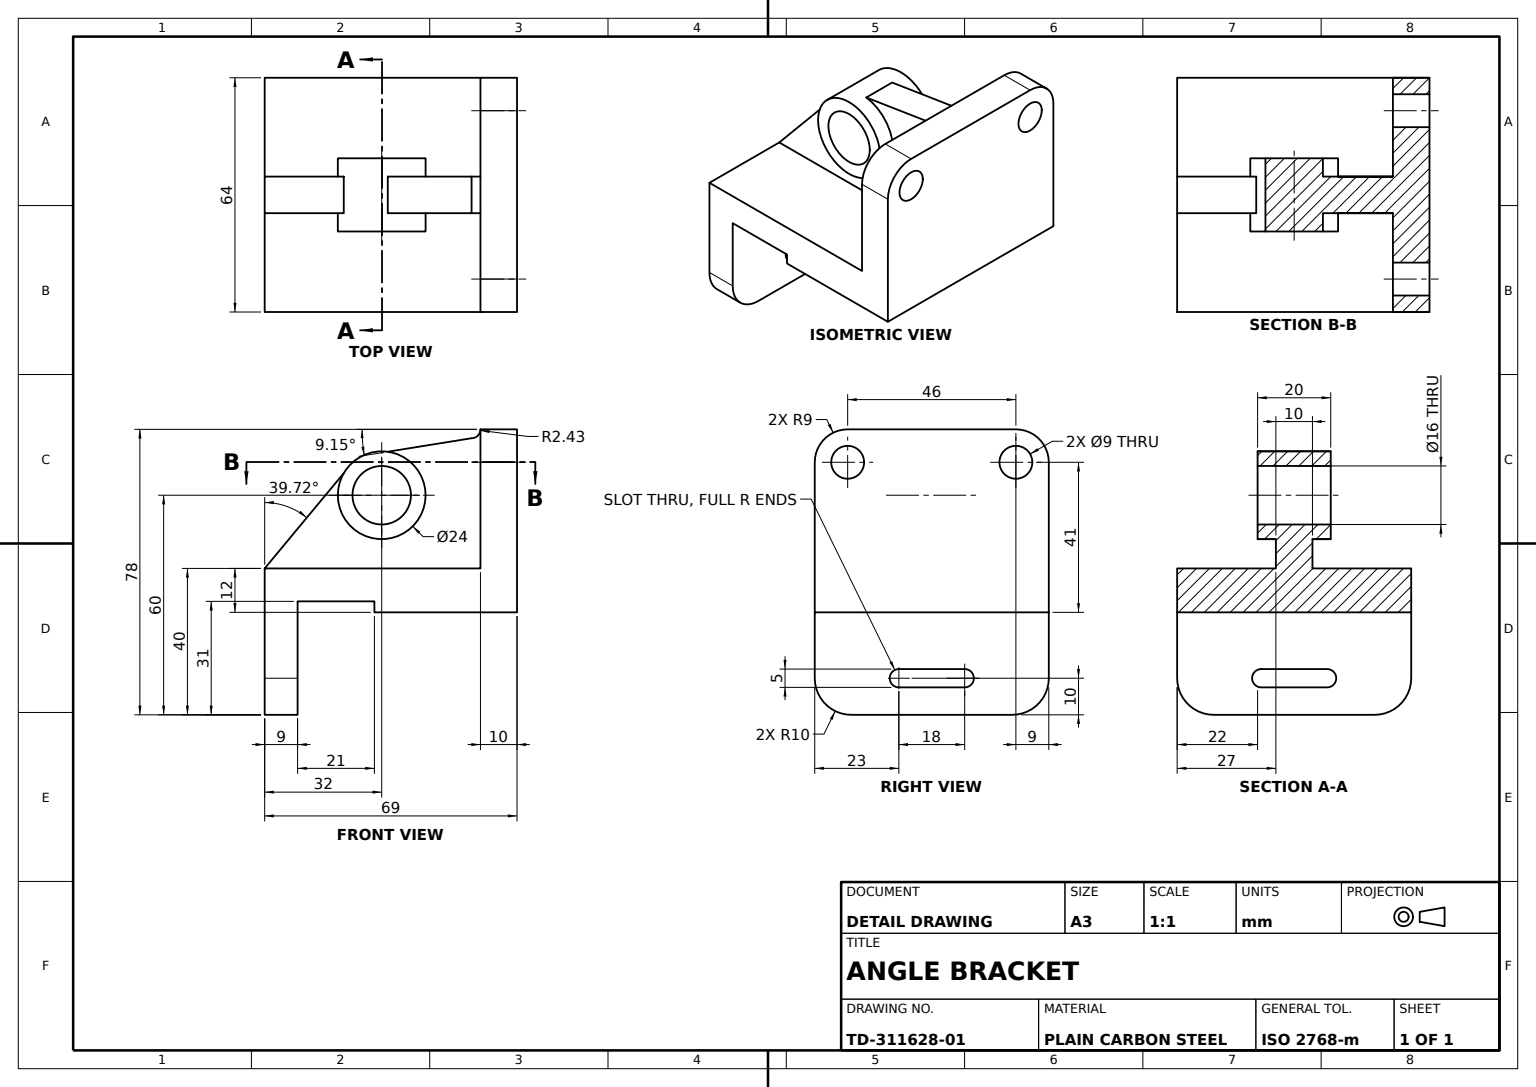
SolidWorks part; units mm, degrees
material "Plain Carbon Steel"
ref_plane "Front Plane" through (0, 0, 0) normal (0, 0, 1) x (1, 0, 0)
ref_plane "Top Plane" through (0, 0, 0) normal (0, 1, 0) x (1, 0, 0)
ref_plane "Right Plane" through (0, 0, 0) normal (1, 0, 0) x (0, 0, -1)
sketch "Back Plate Sketch" plane through (0, 0, 0) normal (0, 0, 1) x (1, 0, 0)
  line L0 (0, 0) -> (0, 41)
  line L1 (9, 50) -> (55, 50)
  line L2 (64, 41) -> (64, 0)
  line L3 (64, 0) -> (0, 0)
  arc A0 (0, 41) -> (9, 50) centre (9, 41) cw
  arc A1 (55, 50) -> (64, 41) centre (55, 41) cw
  dimension "D1" = 9
  dimension "D2" = 9
  dimension "D3" = 41
  dimension "D4" = 41
  dimension "D5" = 64
extrude "Back Plate" add sketch "Back Plate Sketch" along normal blind 10
sketch "Mounting Holes Sketch" plane through (0, 0, 10) normal (0, 0, 1) x (1, 0, 0)
  circle A0 centre (9, 41) radius 4.5
  circle A1 centre (55, 41) radius 4.5
  dimension "D1" = 9
  dimension "D2" = 9
extrude "Mounting Holes 2x" cut sketch "Mounting Holes Sketch" against normal blind 10
sketch "L-Base Profile Sketch" plane through (0, 0, 0) normal (-1, 0, 0) x (0, 0, 1)
  line L0 (0, 0) -> (39, 0)
  line L1 (39, 0) -> (39, 3)
  line L2 (39, 3) -> (60, 3)
  line L3 (60, 3) -> (60, -28)
  line L4 (60, -28) -> (69, -28)
  line L9 (0, 12) -> (69, 12)
  line L10 (0, 41) -> (0, 0) construction
  line L11 (69, 12) -> (69, -28)
  line L12 (0, 12) -> (0, 0)
  dimension "D1" = 39
  dimension "D2" = 9
  dimension "D3" = 9
  dimension "D4" = 21
  dimension "D5" = 40
  dimension "D6" = 12
extrude "L-Base Body" add sketch "L-Base Profile Sketch" against normal blind 64
ref_plane "Hub Mid Plane" through (32, 0, 0) normal (-1, 0, 0) x (0, 0, 1)
sketch "Hub Boss Sketch" plane through (32, 0, 0) normal (-1, 0, 0) x (0, 0, 1)
  line L0 (69, 12) -> (10, 12) construction
  circle A0 centre (37, 32) radius 12
  dimension "D1" = 24
  dimension "D2" = 20
  dimension "D3" = 32
extrude "Hub Boss" add sketch "Hub Boss Sketch" along normal mid plane 20 separate body
sketch "Support Rib Sketch" plane through (32, 0, 0) normal (-1, 0, 0) x (0, 0, 1)
  line L0 (10, 12) -> (69, 12)
  line L1 (10, 12) -> (10, 50)
  line L2 (12.4266, 47.5734) -> (35.3396, 43.8846)
  line L3 (69, 12) -> (44.8306, 41.0929)
  line L4 (44.8306, 41.0929) -> (35.3396, 43.8846)
  arc A0 (10, 50) -> (12.4266, 47.5734) centre (12.4266, 50) ccw
  circle A1 centre (37, 32) radius 12 construction
  dimension "D3" = 2.4266
  dimension "D1" = 29.0929
  dimension "D2" = 23.2081
  dimension "D4" = 9.491
extrude "Support Rib" add sketch "Support Rib Sketch" along normal mid plane 10
sketch "Hub Bore Sketch" plane through (22, 0, 0) normal (-1, 0, 0) x (0, 0, 1)
  circle A0 centre (37, 32) radius 8
  dimension "D1" = 16
extrude "Hub Bore Ø16" cut sketch "Hub Bore Sketch" against normal mid plane 60
sketch "Front Slot Sketch" plane through (0, 0, 69) normal (0, 0, 1) x (1, 0, 0)
  line L0 (0, -28) -> (0, 12) construction
  line L1 (64, -28) -> (64, 12) construction
  line L2 (64, -28) -> (0, -28) construction
  line L3 (23, -15.5) -> (41, -15.5)
  line L4 (41, -20.5) -> (23, -20.5)
  arc A0 (23, -15.5) -> (23, -20.5) centre (23, -18) ccw
  arc A1 (41, -20.5) -> (41, -15.5) centre (41, -18) ccw
  dimension "D4" = 5
  dimension "D5" = 5
  dimension "D1" = 18
  dimension "D2" = 23
  dimension "D3" = 23
  dimension "D6" = 10
  dimension "D7" = 18
  dimension "D8" = 18
extrude "Front Slot" cut sketch "Front Slot Sketch" against normal mid plane 60
fillet "Edge Fillet R10 A" radius 10 1 edges at (0, -28, 64.5)
fillet "Edge Fillet R10 B" radius 10 1 edges at (64, -28, 64.5)
